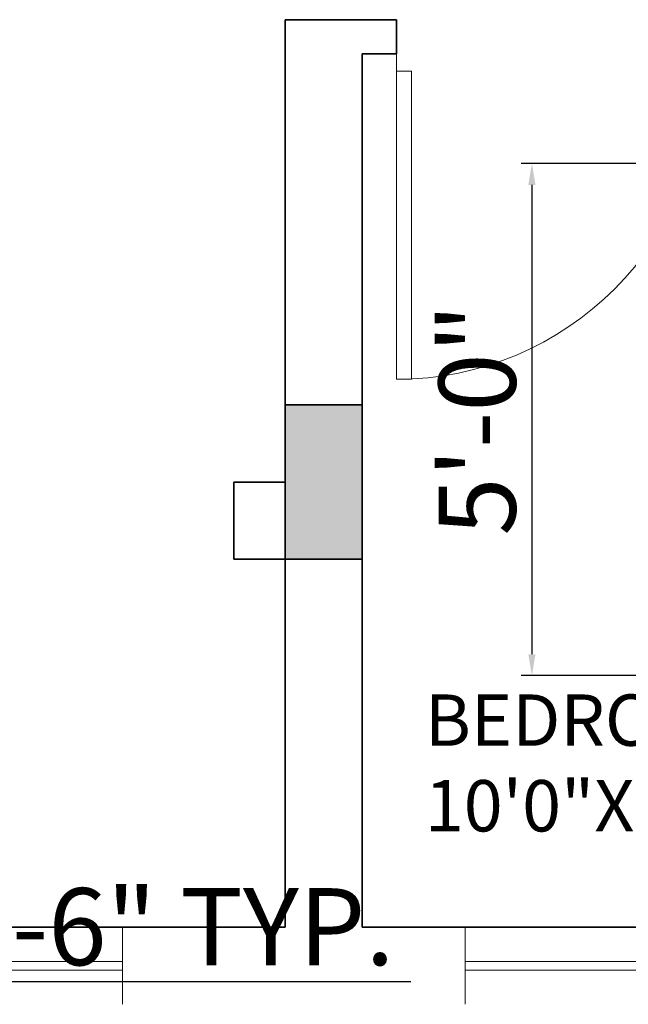
# Model space of a CAD drawing. Units: inches. Extents: x 3321 to 5237, y 11 to 1752.
# Tile 15 of 43: x 4296 to 4367, y 1172 to 1287. Entities that reach past the tile are written whole.
import ezdxf

# ---------------------------------------------------------------- set-up
doc = ezdxf.new("R2010")
doc.units = ezdxf.units.IN
for name, color, linetype, lineweight in [('A-ANNO-DIMS', 2, 'Continuous', 18), ('A-AREA-IDEN', 7, 'Continuous', 18), ('A-COLS', 1, 'Continuous', 35), ('A-DOOR', 4, 'Continuous', 18), ('A-GLAZ', 5, 'Continuous', 18), ('A-WALL', 7, 'Continuous', 35)]:
    doc.layers.add(name, color=color, linetype=linetype, lineweight=lineweight)
doc.styles.get("Standard").update_dxf_attribs({"font": 'arial.ttf'})
doc.dimstyles.new('ISO-25', dxfattribs={"dimtxt": 9, "dimasz": 2.5, "dimexe": 1.25, "dimexo": 0.625, "dimtad": 1, "dimdec": 1, "dimlunit": 3, "dimtxsty": 'Standard', "dimcen": 2.5, "dimclrd": 4, "dimclre": 4, "dimclrt": 256, "dimadec": 0, "dimazin": 0, "dimtfac": 1, "dimtdec": 1, "dimtmove": 0, "dimatfit": 3, "dimfxl": 1, "dimarcsym": 0})

# ---------------------------------------------------------------- blocks, each defined once
blk = doc.blocks.new('*U9')
for p, q in [((-36, 0), (-36, 6)), ((0, 0), (0, 6))]:
    blk.add_line(p, q)
blk.add_lwpolyline([(0, 0), (0, -36), (-1.75, -36), (-1.75, 0)], close=True)
blk.add_arc((0, 0), 36, 180, 270)
blk = doc.blocks.new('COL-9X18-IN')
h = blk.add_hatch(color=256)
h.dxf.hatch_style = 1
h.paths.add_polyline_path([(9, 18), (0, 18), (0, 0), (9, 0)])
blk.add_lwpolyline([(0, 0), (9, 0), (9, 18), (0, 18)], close=True)
blk = doc.blocks.new('WIN-48IN-9IN-WALL')
for p, q in [((0, 0), (0, 9)), ((48, 0), (48, 9)), ((0, 5), (48, 5)), ((0, 4), (48, 4))]:
    blk.add_line(p, q)
blk = doc.blocks.new('*D196')
at = {"layer": 'A-ANNO-DIMS', "color": 4, "lineweight": -2, "transparency": 16777216}
for p, q in [((4368.45, 1270.54), (4354.95, 1270.54)), ((4356.2, 1268.04), (4356.2, 1213.23)), ((4368.45, 1210.73), (4354.95, 1210.73))]:
    blk.add_line(p, q, dxfattribs=at)
at = {"layer": 'A-ANNO-DIMS', "color": 4, "transparency": 16777216}
for points in [[(4355.78, 1268.04), (4356.62, 1268.04), (4356.2, 1270.54)], [(4355.78, 1213.23), (4356.62, 1213.23), (4356.2, 1210.73)]]:
    blk.add_solid(points, dxfattribs=at)
at = {"layer": 'Defpoints', "color": 0, "transparency": 16777216}
for p in [(4369.07, 1270.54), (4356.2, 1210.73), (4369.07, 1210.73)]:
    blk.add_point(p, dxfattribs=at)
at = {"layer": 'A-ANNO-DIMS', "transparency": 16777216, "insert": (4350.98, 1240.63), "char_height": 9, "attachment_point": 5, "rotation": 90}
blk.add_mtext('5\'-0"', dxfattribs=at)
blk = doc.blocks.new('*D215')
at = {"layer": 'A-ANNO-DIMS', "color": 4, "lineweight": -2, "transparency": 16777216}
for p, q in [((4221.54, 1180.71), (4221.54, 1173.77)), ((4263.67, 1180.71), (4263.67, 1173.77)), ((4224.04, 1175.02), (4261.17, 1175.02)), ((4263.67, 1175.02), (4342.06, 1175.02))]:
    blk.add_line(p, q, dxfattribs=at)
at = {"layer": 'A-ANNO-DIMS', "color": 4, "transparency": 16777216}
for points in [[(4224.04, 1175.44), (4224.04, 1174.6), (4221.54, 1175.02)], [(4261.17, 1175.44), (4261.17, 1174.6), (4263.67, 1175.02)]]:
    blk.add_solid(points, dxfattribs=at)
at = {"layer": 'Defpoints', "color": 0, "transparency": 16777216}
for p in [(4221.54, 1181.34), (4263.67, 1181.34), (4263.67, 1175.02)]:
    blk.add_point(p, dxfattribs=at)
at = {"layer": 'A-ANNO-DIMS', "transparency": 16777216, "insert": (4304.12, 1180.24), "char_height": 9, "attachment_point": 5}
blk.add_mtext('TV 3\'-6" TYP.', dxfattribs=at)

msp = doc.modelspace()

# ---------------------------------------------------------------- linework, layer by layer
at = {"layer": 'A-WALL'}
for p, q in [((4327.39, 1287.34), (4327.39, 1233.34)), ((4327.39, 1287.34), (4340.39, 1287.34)), ((4340.39, 1287.34), (4340.39, 1283.34)), ((4336.39, 1283.34), (4336.39, 1181.34)), ((4336.39, 1283.34), (4340.39, 1283.34)), ((4321.39, 1233.34), (4327.39, 1233.34)), ((4321.39, 1233.34), (4321.39, 1224.34)), ((4321.39, 1224.34), (4327.39, 1224.34)), ((4327.39, 1224.34), (4327.39, 1181.34)), ((4126.39, 1181.34), (4327.39, 1181.34)), ((4336.39, 1181.34), (4456.39, 1181.34))]:
    msp.add_line(p, q, dxfattribs=at)

# ---------------------------------------------------------------- block references
at = {"layer": 'A-COLS', "rotation": 180}
msp.add_blockref('COL-9X18-IN', (4336.39, 1242.34), dxfattribs=at)
at = {"layer": 'A-DOOR', "xscale": -1}
msp.add_blockref('*U9', (4340.39, 1281.34), dxfattribs=at)
at = {"layer": 'A-GLAZ'}
for p in [(4260.39, 1172.34), (4348.39, 1172.34)]:
    msp.add_blockref('WIN-48IN-9IN-WALL', p, dxfattribs=at)

# ---------------------------------------------------------------- texts
at = {"layer": 'A-AREA-IDEN', "insert": (4343.7, 1208.53), "char_height": 6, "attachment_point": 1}
msp.add_mtext_dynamic_manual_height_columns('BEDROOM\\P10\'0"X8\'6"', width=97.3114, gutter_width=25, heights=[0], dxfattribs=at)

# ---------------------------------------------------------------- dimensions: what is measured, and where the dimension line sits
at = {"layer": 'A-ANNO-DIMS'}
dim = msp.add_linear_dim(base=(4356.2, 1210.73), p1=(4369.07, 1270.54), p2=(4369.07, 1210.73), angle=270, dimstyle='ISO-25', override={"dimdec": 1, "dimlfac": 1, "dimrnd": 0, "dimzin": 1, "dimdsep": 46, "dimlunit": 4, "dimfrac": 2}, dxfattribs=at)
dim.commit()
dim.dimension.update_dxf_attribs({"geometry": '*D196', "text_midpoint": (4350.98, 1240.63)})
dim = msp.add_linear_dim(base=(4263.67, 1175.02), p1=(4221.54, 1181.34), p2=(4263.67, 1181.34), text='TV <> TYP.', dimstyle='ISO-25', override={"dimdec": 1, "dimlfac": 1, "dimrnd": 0, "dimzin": 1, "dimdsep": 46, "dimlunit": 4, "dimfrac": 2}, dxfattribs=at)
dim.commit()
dim.dimension.update_dxf_attribs({"geometry": '*D215', "text_midpoint": (4304.12, 1180.24)})

doc.saveas('drawing.dxf')
